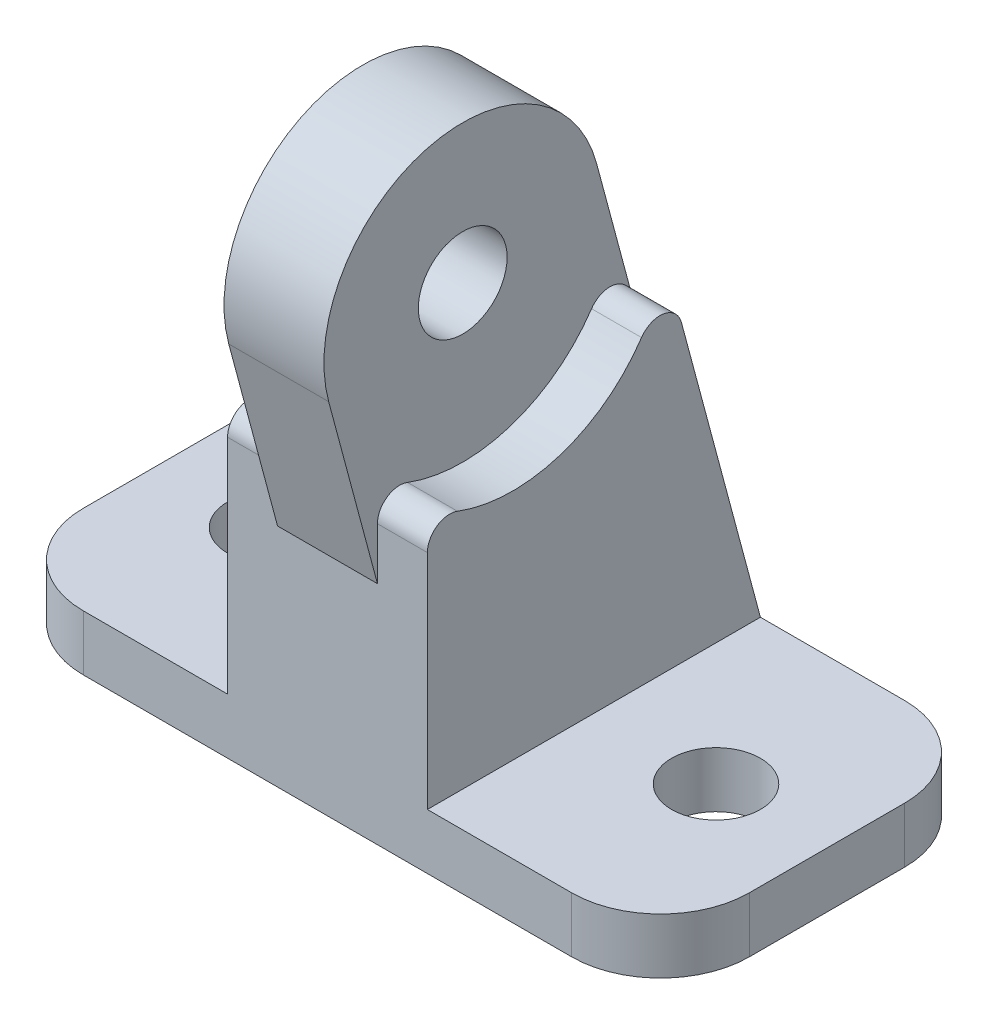
ISO-10303-21;
HEADER;
FILE_DESCRIPTION(('STEP AP214'),'2;1');
FILE_NAME('part.step','',(''),(''),'','','');
FILE_SCHEMA(('AUTOMOTIVE_DESIGN { 1 0 10303 214 1 1 1 1 }'));
ENDSEC;
DATA;
#1=APPLICATION_CONTEXT('core data for automotive mechanical design processes');
#2=APPLICATION_PROTOCOL_DEFINITION('international standard','automotive_design',2000,#1);
#3=PRODUCT_CONTEXT('',#1,'mechanical');
#4=PRODUCT('Part','Part','',(#3));
#5=PRODUCT_RELATED_PRODUCT_CATEGORY('part','',(#4));
#6=PRODUCT_DEFINITION_FORMATION('','',#4);
#7=PRODUCT_DEFINITION_CONTEXT('part definition',#1,'design');
#8=PRODUCT_DEFINITION('design','',#6,#7);
#9=PRODUCT_DEFINITION_SHAPE('','',#8);
#10=(LENGTH_UNIT() NAMED_UNIT(*) SI_UNIT(.MILLI.,.METRE.));
#11=(NAMED_UNIT(*) PLANE_ANGLE_UNIT() SI_UNIT($,.RADIAN.));
#12=(NAMED_UNIT(*) SI_UNIT($,.STERADIAN.) SOLID_ANGLE_UNIT());
#13=UNCERTAINTY_MEASURE_WITH_UNIT(LENGTH_MEASURE(1.E-05),#10,'distance_accuracy_value','');
#14=(GEOMETRIC_REPRESENTATION_CONTEXT(3) GLOBAL_UNCERTAINTY_ASSIGNED_CONTEXT((#13)) GLOBAL_UNIT_ASSIGNED_CONTEXT((#10,
#11,#12)) REPRESENTATION_CONTEXT('',''));
#15=CARTESIAN_POINT('',(0.,0.,0.));
#16=DIRECTION('',(0.,0.,1.));
#17=DIRECTION('',(1.,0.,0.));
#18=AXIS2_PLACEMENT_3D('',#15,#16,#17);
#19=CARTESIAN_POINT('',(-9.,0.,0.));
#20=DIRECTION('',(1.,0.,0.));
#21=DIRECTION('',(0.,0.,-1.));
#22=AXIS2_PLACEMENT_3D('',#19,#20,#21);
#23=PLANE('',#22);
#24=DIRECTION('',(0.,1.,0.));
#25=VECTOR('',#24,1.);
#26=CARTESIAN_POINT('',(-9.,0.,15.));
#27=LINE('',#26,#25);
#28=CARTESIAN_POINT('',(-9.,5.,15.));
#29=VERTEX_POINT('',#28);
#30=CARTESIAN_POINT('',(-9.,25.0424528800157,15.));
#31=VERTEX_POINT('',#30);
#32=EDGE_CURVE('E288',#29,#31,#27,.T.);
#33=ORIENTED_EDGE('',*,*,#32,.T.);
#34=CARTESIAN_POINT('',(-9.,25.0424528800157,13.));
#35=DIRECTION('',(1.,0.,0.));
#36=DIRECTION('',(0.,0.,-1.));
#37=AXIS2_PLACEMENT_3D('',#34,#35,#36);
#38=CIRCLE('',#37,2.);
#39=CARTESIAN_POINT('',(-9.,26.9121462700137,12.2898967487769));
#40=VERTEX_POINT('',#39);
#41=EDGE_CURVE('E277',#40,#31,#38,.T.);
#42=ORIENTED_EDGE('',*,*,#41,.F.);
#43=CARTESIAN_POINT('',(-9.,40.,7.31917399021508));
#44=DIRECTION('',(1.,0.,0.));
#45=DIRECTION('',(0.,0.,-1.));
#46=AXIS2_PLACEMENT_3D('',#43,#44,#45);
#47=CIRCLE('',#46,14.);
#48=CARTESIAN_POINT('',(-9.,32.1742368297092,-4.28933283893913));
#49=VERTEX_POINT('',#48);
#50=EDGE_CURVE('E273',#49,#40,#47,.F.);
#51=ORIENTED_EDGE('',*,*,#50,.F.);
#52=CARTESIAN_POINT('',(-9.,31.0562706625248,-5.94769095738974));
#53=DIRECTION('',(1.,0.,0.));
#54=DIRECTION('',(0.,0.,-1.));
#55=AXIS2_PLACEMENT_3D('',#52,#53,#54);
#56=CIRCLE('',#55,2.);
#57=CARTESIAN_POINT('',(-9.,31.5739087527298,-7.87954260996788));
#58=VERTEX_POINT('',#57);
#59=EDGE_CURVE('E275',#58,#49,#56,.T.);
#60=ORIENTED_EDGE('',*,*,#59,.F.);
#61=DIRECTION('',(0.,0.96592582628907,0.258819045102515));
#62=VECTOR('',#61,1.);
#63=CARTESIAN_POINT('',(-9.,4.0849364905388,-15.2451905283833));
#64=LINE('',#63,#62);
#65=CARTESIAN_POINT('',(-9.,5.,-15.));
#66=VERTEX_POINT('',#65);
#67=EDGE_CURVE('E236',#66,#58,#64,.T.);
#68=ORIENTED_EDGE('',*,*,#67,.F.);
#69=DIRECTION('',(0.,0.,-1.));
#70=VECTOR('',#69,1.);
#71=CARTESIAN_POINT('',(-9.,5.,0.));
#72=LINE('',#71,#70);
#73=EDGE_CURVE('E100',#29,#66,#72,.T.);
#74=ORIENTED_EDGE('',*,*,#73,.F.);
#75=EDGE_LOOP('',(#33,#42,#51,#60,#68,#74));
#76=FACE_BOUND('',#75,.T.);
#77=ADVANCED_FACE('F71',(#76),#23,.F.);
#78=CARTESIAN_POINT('',(9.,0.,0.));
#79=DIRECTION('',(1.,0.,0.));
#80=DIRECTION('',(0.,0.,-1.));
#81=AXIS2_PLACEMENT_3D('',#78,#79,#80);
#82=PLANE('',#81);
#83=CARTESIAN_POINT('',(9.,25.0424528800157,13.));
#84=DIRECTION('',(1.,0.,0.));
#85=DIRECTION('',(0.,0.,-1.));
#86=AXIS2_PLACEMENT_3D('',#83,#84,#85);
#87=CIRCLE('',#86,2.);
#88=CARTESIAN_POINT('',(9.,26.9121462700137,12.2898967487769));
#89=VERTEX_POINT('',#88);
#90=CARTESIAN_POINT('',(9.,25.0424528800157,15.));
#91=VERTEX_POINT('',#90);
#92=EDGE_CURVE('E13',#89,#91,#87,.T.);
#93=ORIENTED_EDGE('',*,*,#92,.T.);
#94=DIRECTION('',(0.,1.,0.));
#95=VECTOR('',#94,1.);
#96=CARTESIAN_POINT('',(9.,0.,15.));
#97=LINE('',#96,#95);
#98=CARTESIAN_POINT('',(9.,5.,15.));
#99=VERTEX_POINT('',#98);
#100=EDGE_CURVE('E285',#99,#91,#97,.T.);
#101=ORIENTED_EDGE('',*,*,#100,.F.);
#102=DIRECTION('',(0.,0.,-1.));
#103=VECTOR('',#102,1.);
#104=CARTESIAN_POINT('',(9.,5.,0.));
#105=LINE('',#104,#103);
#106=CARTESIAN_POINT('',(9.,5.,-15.));
#107=VERTEX_POINT('',#106);
#108=EDGE_CURVE('E282',#99,#107,#105,.T.);
#109=ORIENTED_EDGE('',*,*,#108,.T.);
#110=DIRECTION('',(0.,0.96592582628907,0.258819045102515));
#111=VECTOR('',#110,1.);
#112=CARTESIAN_POINT('',(9.,4.0849364905388,-15.2451905283833));
#113=LINE('',#112,#111);
#114=CARTESIAN_POINT('',(9.,31.5739087527298,-7.87954260996788));
#115=VERTEX_POINT('',#114);
#116=EDGE_CURVE('E276',#107,#115,#113,.T.);
#117=ORIENTED_EDGE('',*,*,#116,.T.);
#118=CARTESIAN_POINT('',(9.,31.0562706625248,-5.94769095738974));
#119=DIRECTION('',(1.,0.,0.));
#120=DIRECTION('',(0.,0.,-1.));
#121=AXIS2_PLACEMENT_3D('',#118,#119,#120);
#122=CIRCLE('',#121,2.);
#123=CARTESIAN_POINT('',(9.,32.1742368297092,-4.28933283893913));
#124=VERTEX_POINT('',#123);
#125=EDGE_CURVE('E373',#115,#124,#122,.T.);
#126=ORIENTED_EDGE('',*,*,#125,.T.);
#127=CARTESIAN_POINT('',(9.,40.,7.31917399021508));
#128=DIRECTION('',(1.,0.,0.));
#129=DIRECTION('',(0.,0.,-1.));
#130=AXIS2_PLACEMENT_3D('',#127,#128,#129);
#131=CIRCLE('',#130,14.);
#132=EDGE_CURVE('E81',#124,#89,#131,.F.);
#133=ORIENTED_EDGE('',*,*,#132,.T.);
#134=EDGE_LOOP('',(#93,#101,#109,#117,#126,#133));
#135=FACE_BOUND('',#134,.T.);
#136=ADVANCED_FACE('F378',(#135),#82,.T.);
#137=CARTESIAN_POINT('',(-22.,5.,7.));
#138=DIRECTION('',(0.,1.,0.));
#139=DIRECTION('',(0.,0.,1.));
#140=AXIS2_PLACEMENT_3D('',#137,#138,#139);
#141=PLANE('',#140);
#142=CARTESIAN_POINT('',(-20.,5.,0.));
#143=DIRECTION('',(0.,1.,0.));
#144=DIRECTION('',(0.,0.,1.));
#145=AXIS2_PLACEMENT_3D('',#142,#143,#144);
#146=CIRCLE('',#145,4.);
#147=CARTESIAN_POINT('',(-20.,5.,4.));
#148=VERTEX_POINT('',#147);
#149=EDGE_CURVE('E306',#148,#148,#146,.T.);
#150=ORIENTED_EDGE('',*,*,#149,.F.);
#151=EDGE_LOOP('',(#150));
#152=FACE_BOUND('',#151,.T.);
#153=DIRECTION('',(1.,0.,0.));
#154=VECTOR('',#153,1.);
#155=CARTESIAN_POINT('',(-22.,5.,15.));
#156=LINE('',#155,#154);
#157=CARTESIAN_POINT('',(-22.,5.,15.));
#158=VERTEX_POINT('',#157);
#159=EDGE_CURVE('E317',#158,#29,#156,.T.);
#160=ORIENTED_EDGE('',*,*,#159,.T.);
#161=ORIENTED_EDGE('',*,*,#73,.T.);
#162=DIRECTION('',(-1.,0.,0.));
#163=VECTOR('',#162,1.);
#164=CARTESIAN_POINT('',(-22.,5.,-15.));
#165=LINE('',#164,#163);
#166=CARTESIAN_POINT('',(-22.,5.,-15.));
#167=VERTEX_POINT('',#166);
#168=EDGE_CURVE('E330',#66,#167,#165,.T.);
#169=ORIENTED_EDGE('',*,*,#168,.T.);
#170=CARTESIAN_POINT('',(-22.,5.,-7.));
#171=DIRECTION('',(0.,1.,0.));
#172=DIRECTION('',(0.,0.,1.));
#173=AXIS2_PLACEMENT_3D('',#170,#171,#172);
#174=CIRCLE('',#173,8.);
#175=CARTESIAN_POINT('',(-30.,5.,-6.99999999999994));
#176=VERTEX_POINT('',#175);
#177=EDGE_CURVE('E329',#167,#176,#174,.T.);
#178=ORIENTED_EDGE('',*,*,#177,.T.);
#179=DIRECTION('',(0.,0.,1.));
#180=VECTOR('',#179,1.);
#181=CARTESIAN_POINT('',(-30.,5.,-6.99999999999994));
#182=LINE('',#181,#180);
#183=CARTESIAN_POINT('',(-30.,5.,6.99999999999995));
#184=VERTEX_POINT('',#183);
#185=EDGE_CURVE('E335',#176,#184,#182,.T.);
#186=ORIENTED_EDGE('',*,*,#185,.T.);
#187=CARTESIAN_POINT('',(-22.,5.,7.));
#188=DIRECTION('',(0.,1.,0.));
#189=DIRECTION('',(0.,0.,1.));
#190=AXIS2_PLACEMENT_3D('',#187,#188,#189);
#191=CIRCLE('',#190,8.);
#192=EDGE_CURVE('E314',#184,#158,#191,.T.);
#193=ORIENTED_EDGE('',*,*,#192,.T.);
#194=EDGE_LOOP('',(#160,#161,#169,#178,#186,#193));
#195=FACE_BOUND('',#194,.T.);
#196=ADVANCED_FACE('F434',(#152,#195),#141,.T.);
#197=ORIENTED_EDGE('',*,*,#108,.F.);
#198=CARTESIAN_POINT('',(21.9999999999999,5.,15.));
#199=VERTEX_POINT('',#198);
#200=EDGE_CURVE('E320',#99,#199,#156,.T.);
#201=ORIENTED_EDGE('',*,*,#200,.T.);
#202=CARTESIAN_POINT('',(22.,5.,7.));
#203=DIRECTION('',(0.,1.,0.));
#204=DIRECTION('',(0.,0.,1.));
#205=AXIS2_PLACEMENT_3D('',#202,#203,#204);
#206=CIRCLE('',#205,8.);
#207=CARTESIAN_POINT('',(30.,5.,6.99999999999995));
#208=VERTEX_POINT('',#207);
#209=EDGE_CURVE('E321',#199,#208,#206,.T.);
#210=ORIENTED_EDGE('',*,*,#209,.T.);
#211=DIRECTION('',(0.,0.,-1.));
#212=VECTOR('',#211,1.);
#213=CARTESIAN_POINT('',(30.,5.,-6.99999999999994));
#214=LINE('',#213,#212);
#215=CARTESIAN_POINT('',(30.,5.,-6.99999999999994));
#216=VERTEX_POINT('',#215);
#217=EDGE_CURVE('E323',#208,#216,#214,.T.);
#218=ORIENTED_EDGE('',*,*,#217,.T.);
#219=CARTESIAN_POINT('',(22.,5.,-7.));
#220=DIRECTION('',(0.,1.,0.));
#221=DIRECTION('',(0.,0.,-1.));
#222=AXIS2_PLACEMENT_3D('',#219,#220,#221);
#223=CIRCLE('',#222,8.);
#224=CARTESIAN_POINT('',(21.9999999999999,5.,-15.));
#225=VERTEX_POINT('',#224);
#226=EDGE_CURVE('E324',#216,#225,#223,.T.);
#227=ORIENTED_EDGE('',*,*,#226,.T.);
#228=EDGE_CURVE('E327',#225,#107,#165,.T.);
#229=ORIENTED_EDGE('',*,*,#228,.T.);
#230=EDGE_LOOP('',(#197,#201,#210,#218,#227,#229));
#231=FACE_BOUND('',#230,.T.);
#232=CARTESIAN_POINT('',(20.,5.,0.));
#233=DIRECTION('',(0.,1.,0.));
#234=DIRECTION('',(0.,0.,1.));
#235=AXIS2_PLACEMENT_3D('',#232,#233,#234);
#236=CIRCLE('',#235,4.);
#237=CARTESIAN_POINT('',(20.,5.,3.99999999999999));
#238=VERTEX_POINT('',#237);
#239=EDGE_CURVE('E301',#238,#238,#236,.T.);
#240=ORIENTED_EDGE('',*,*,#239,.F.);
#241=EDGE_LOOP('',(#240));
#242=FACE_BOUND('',#241,.T.);
#243=ADVANCED_FACE('F451',(#231,#242),#141,.T.);
#244=CARTESIAN_POINT('',(-22.,0.,7.));
#245=DIRECTION('',(0.,1.,0.));
#246=DIRECTION('',(0.,0.,1.));
#247=AXIS2_PLACEMENT_3D('',#244,#245,#246);
#248=PLANE('',#247);
#249=CARTESIAN_POINT('',(-22.,0.,7.));
#250=DIRECTION('',(0.,1.,0.));
#251=DIRECTION('',(0.,0.,1.));
#252=AXIS2_PLACEMENT_3D('',#249,#250,#251);
#253=CIRCLE('',#252,8.);
#254=CARTESIAN_POINT('',(-30.,0.,6.99999999999995));
#255=VERTEX_POINT('',#254);
#256=CARTESIAN_POINT('',(-22.,0.,15.));
#257=VERTEX_POINT('',#256);
#258=EDGE_CURVE('E313',#255,#257,#253,.T.);
#259=ORIENTED_EDGE('',*,*,#258,.F.);
#260=DIRECTION('',(0.,0.,1.));
#261=VECTOR('',#260,1.);
#262=CARTESIAN_POINT('',(-30.,0.,-6.99999999999994));
#263=LINE('',#262,#261);
#264=CARTESIAN_POINT('',(-30.,0.,-6.99999999999994));
#265=VERTEX_POINT('',#264);
#266=EDGE_CURVE('E318',#265,#255,#263,.T.);
#267=ORIENTED_EDGE('',*,*,#266,.F.);
#268=CARTESIAN_POINT('',(-22.,0.,-7.));
#269=DIRECTION('',(0.,1.,0.));
#270=DIRECTION('',(0.,0.,1.));
#271=AXIS2_PLACEMENT_3D('',#268,#269,#270);
#272=CIRCLE('',#271,8.);
#273=CARTESIAN_POINT('',(-22.,0.,-15.));
#274=VERTEX_POINT('',#273);
#275=EDGE_CURVE('E350',#274,#265,#272,.T.);
#276=ORIENTED_EDGE('',*,*,#275,.F.);
#277=DIRECTION('',(-1.,0.,0.));
#278=VECTOR('',#277,1.);
#279=CARTESIAN_POINT('',(-22.,0.,-15.));
#280=LINE('',#279,#278);
#281=CARTESIAN_POINT('',(21.9999999999999,0.,-15.));
#282=VERTEX_POINT('',#281);
#283=EDGE_CURVE('E342',#282,#274,#280,.T.);
#284=ORIENTED_EDGE('',*,*,#283,.F.);
#285=CARTESIAN_POINT('',(22.,0.,-7.));
#286=DIRECTION('',(0.,1.,0.));
#287=DIRECTION('',(0.,0.,-1.));
#288=AXIS2_PLACEMENT_3D('',#285,#286,#287);
#289=CIRCLE('',#288,8.);
#290=CARTESIAN_POINT('',(30.,0.,-6.99999999999994));
#291=VERTEX_POINT('',#290);
#292=EDGE_CURVE('E345',#291,#282,#289,.T.);
#293=ORIENTED_EDGE('',*,*,#292,.F.);
#294=DIRECTION('',(0.,0.,-1.));
#295=VECTOR('',#294,1.);
#296=CARTESIAN_POINT('',(30.,0.,-6.99999999999994));
#297=LINE('',#296,#295);
#298=CARTESIAN_POINT('',(30.,0.,6.99999999999995));
#299=VERTEX_POINT('',#298);
#300=EDGE_CURVE('E344',#299,#291,#297,.T.);
#301=ORIENTED_EDGE('',*,*,#300,.F.);
#302=CARTESIAN_POINT('',(22.,0.,7.));
#303=DIRECTION('',(0.,1.,0.));
#304=DIRECTION('',(0.,0.,1.));
#305=AXIS2_PLACEMENT_3D('',#302,#303,#304);
#306=CIRCLE('',#305,8.);
#307=CARTESIAN_POINT('',(21.9999999999999,0.,15.));
#308=VERTEX_POINT('',#307);
#309=EDGE_CURVE('E337',#308,#299,#306,.T.);
#310=ORIENTED_EDGE('',*,*,#309,.F.);
#311=DIRECTION('',(1.,0.,0.));
#312=VECTOR('',#311,1.);
#313=CARTESIAN_POINT('',(-22.,0.,15.));
#314=LINE('',#313,#312);
#315=EDGE_CURVE('E340',#257,#308,#314,.T.);
#316=ORIENTED_EDGE('',*,*,#315,.F.);
#317=EDGE_LOOP('',(#259,#267,#276,#284,#293,#301,#310,#316));
#318=FACE_BOUND('',#317,.T.);
#319=CARTESIAN_POINT('',(-20.,0.,0.));
#320=DIRECTION('',(0.,1.,0.));
#321=DIRECTION('',(0.,0.,1.));
#322=AXIS2_PLACEMENT_3D('',#319,#320,#321);
#323=CIRCLE('',#322,4.);
#324=CARTESIAN_POINT('',(-20.,0.,4.));
#325=VERTEX_POINT('',#324);
#326=EDGE_CURVE('E302',#325,#325,#323,.T.);
#327=ORIENTED_EDGE('',*,*,#326,.T.);
#328=EDGE_LOOP('',(#327));
#329=FACE_BOUND('',#328,.T.);
#330=CARTESIAN_POINT('',(20.,0.,0.));
#331=DIRECTION('',(0.,1.,0.));
#332=DIRECTION('',(0.,0.,1.));
#333=AXIS2_PLACEMENT_3D('',#330,#331,#332);
#334=CIRCLE('',#333,4.);
#335=CARTESIAN_POINT('',(20.,0.,3.99999999999999));
#336=VERTEX_POINT('',#335);
#337=EDGE_CURVE('E304',#336,#336,#334,.T.);
#338=ORIENTED_EDGE('',*,*,#337,.T.);
#339=EDGE_LOOP('',(#338));
#340=FACE_BOUND('',#339,.T.);
#341=ADVANCED_FACE('F445',(#318,#329,#340),#248,.F.);
#342=CARTESIAN_POINT('',(-22.,5.,7.));
#343=DIRECTION('',(0.,-1.,0.));
#344=DIRECTION('',(0.,0.,-1.));
#345=AXIS2_PLACEMENT_3D('',#342,#343,#344);
#346=CYLINDRICAL_SURFACE('',#345,8.);
#347=ORIENTED_EDGE('',*,*,#258,.T.);
#348=DIRECTION('',(0.,-1.,0.));
#349=VECTOR('',#348,1.);
#350=CARTESIAN_POINT('',(-22.,5.,15.));
#351=LINE('',#350,#349);
#352=EDGE_CURVE('E367',#158,#257,#351,.T.);
#353=ORIENTED_EDGE('',*,*,#352,.F.);
#354=ORIENTED_EDGE('',*,*,#192,.F.);
#355=DIRECTION('',(0.,-1.,0.));
#356=VECTOR('',#355,1.);
#357=CARTESIAN_POINT('',(-30.,5.,6.99999999999995));
#358=LINE('',#357,#356);
#359=EDGE_CURVE('E331',#184,#255,#358,.T.);
#360=ORIENTED_EDGE('',*,*,#359,.T.);
#361=EDGE_LOOP('',(#347,#353,#354,#360));
#362=FACE_BOUND('',#361,.T.);
#363=ADVANCED_FACE('F73',(#362),#346,.T.);
#364=CARTESIAN_POINT('',(-22.,5.,15.));
#365=DIRECTION('',(0.,0.,-1.));
#366=DIRECTION('',(-1.,0.,0.));
#367=AXIS2_PLACEMENT_3D('',#364,#365,#366);
#368=PLANE('',#367);
#369=ORIENTED_EDGE('',*,*,#315,.T.);
#370=DIRECTION('',(0.,-1.,0.));
#371=VECTOR('',#370,1.);
#372=CARTESIAN_POINT('',(21.9999999999999,5.,15.));
#373=LINE('',#372,#371);
#374=EDGE_CURVE('E370',#199,#308,#373,.T.);
#375=ORIENTED_EDGE('',*,*,#374,.F.);
#376=ORIENTED_EDGE('',*,*,#200,.F.);
#377=ORIENTED_EDGE('',*,*,#100,.T.);
#378=DIRECTION('',(1.,0.,0.));
#379=VECTOR('',#378,1.);
#380=CARTESIAN_POINT('',(-42.4219732605604,25.0424528800157,15.));
#381=LINE('',#380,#379);
#382=CARTESIAN_POINT('',(4.5,25.0424528800157,15.));
#383=VERTEX_POINT('',#382);
#384=EDGE_CURVE('E234',#383,#91,#381,.T.);
#385=ORIENTED_EDGE('',*,*,#384,.F.);
#386=DIRECTION('',(0.,-1.,0.));
#387=VECTOR('',#386,1.);
#388=CARTESIAN_POINT('',(4.5,20.36894159816,15.));
#389=LINE('',#388,#387);
#390=CARTESIAN_POINT('',(4.5,20.36894159816,15.));
#391=VERTEX_POINT('',#390);
#392=EDGE_CURVE('E242',#383,#391,#389,.T.);
#393=ORIENTED_EDGE('',*,*,#392,.T.);
#394=DIRECTION('',(-1.,0.,0.));
#395=VECTOR('',#394,1.);
#396=CARTESIAN_POINT('',(9.,20.36894159816,15.));
#397=LINE('',#396,#395);
#398=CARTESIAN_POINT('',(-4.5,20.36894159816,15.));
#399=VERTEX_POINT('',#398);
#400=EDGE_CURVE('E291',#391,#399,#397,.T.);
#401=ORIENTED_EDGE('',*,*,#400,.T.);
#402=DIRECTION('',(0.,1.,0.));
#403=VECTOR('',#402,1.);
#404=CARTESIAN_POINT('',(-4.5,20.36894159816,15.));
#405=LINE('',#404,#403);
#406=CARTESIAN_POINT('',(-4.5,25.0424528800157,15.));
#407=VERTEX_POINT('',#406);
#408=EDGE_CURVE('E415',#399,#407,#405,.T.);
#409=ORIENTED_EDGE('',*,*,#408,.T.);
#410=DIRECTION('',(-1.,0.,0.));
#411=VECTOR('',#410,1.);
#412=CARTESIAN_POINT('',(42.4219732605604,25.0424528800157,15.));
#413=LINE('',#412,#411);
#414=EDGE_CURVE('E418',#407,#31,#413,.T.);
#415=ORIENTED_EDGE('',*,*,#414,.T.);
#416=ORIENTED_EDGE('',*,*,#32,.F.);
#417=ORIENTED_EDGE('',*,*,#159,.F.);
#418=ORIENTED_EDGE('',*,*,#352,.T.);
#419=EDGE_LOOP('',(#369,#375,#376,#377,#385,#393,#401,#409,#415,#416,#417,#418));
#420=FACE_BOUND('',#419,.T.);
#421=ADVANCED_FACE('F396',(#420),#368,.F.);
#422=CARTESIAN_POINT('',(22.,5.,7.));
#423=DIRECTION('',(0.,-1.,0.));
#424=DIRECTION('',(0.,0.,-1.));
#425=AXIS2_PLACEMENT_3D('',#422,#423,#424);
#426=CYLINDRICAL_SURFACE('',#425,8.);
#427=ORIENTED_EDGE('',*,*,#309,.T.);
#428=DIRECTION('',(0.,-1.,0.));
#429=VECTOR('',#428,1.);
#430=CARTESIAN_POINT('',(30.,5.,6.99999999999995));
#431=LINE('',#430,#429);
#432=EDGE_CURVE('E365',#208,#299,#431,.T.);
#433=ORIENTED_EDGE('',*,*,#432,.F.);
#434=ORIENTED_EDGE('',*,*,#209,.F.);
#435=ORIENTED_EDGE('',*,*,#374,.T.);
#436=EDGE_LOOP('',(#427,#433,#434,#435));
#437=FACE_BOUND('',#436,.T.);
#438=ADVANCED_FACE('F447',(#437),#426,.T.);
#439=CARTESIAN_POINT('',(30.,5.,-6.99999999999994));
#440=DIRECTION('',(-1.,0.,0.));
#441=DIRECTION('',(0.,0.,1.));
#442=AXIS2_PLACEMENT_3D('',#439,#440,#441);
#443=PLANE('',#442);
#444=ORIENTED_EDGE('',*,*,#300,.T.);
#445=DIRECTION('',(0.,-1.,0.));
#446=VECTOR('',#445,1.);
#447=CARTESIAN_POINT('',(30.,5.,-6.99999999999994));
#448=LINE('',#447,#446);
#449=EDGE_CURVE('E363',#216,#291,#448,.T.);
#450=ORIENTED_EDGE('',*,*,#449,.F.);
#451=ORIENTED_EDGE('',*,*,#217,.F.);
#452=ORIENTED_EDGE('',*,*,#432,.T.);
#453=EDGE_LOOP('',(#444,#450,#451,#452));
#454=FACE_BOUND('',#453,.T.);
#455=ADVANCED_FACE('F456',(#454),#443,.F.);
#456=CARTESIAN_POINT('',(22.,5.,-7.));
#457=DIRECTION('',(0.,-1.,0.));
#458=DIRECTION('',(0.,0.,-1.));
#459=AXIS2_PLACEMENT_3D('',#456,#457,#458);
#460=CYLINDRICAL_SURFACE('',#459,8.);
#461=ORIENTED_EDGE('',*,*,#292,.T.);
#462=DIRECTION('',(0.,-1.,0.));
#463=VECTOR('',#462,1.);
#464=CARTESIAN_POINT('',(21.9999999999999,5.,-15.));
#465=LINE('',#464,#463);
#466=EDGE_CURVE('E360',#225,#282,#465,.T.);
#467=ORIENTED_EDGE('',*,*,#466,.F.);
#468=ORIENTED_EDGE('',*,*,#226,.F.);
#469=ORIENTED_EDGE('',*,*,#449,.T.);
#470=EDGE_LOOP('',(#461,#467,#468,#469));
#471=FACE_BOUND('',#470,.T.);
#472=ADVANCED_FACE('F463',(#471),#460,.T.);
#473=CARTESIAN_POINT('',(-22.,5.,-15.));
#474=DIRECTION('',(0.,0.,1.));
#475=DIRECTION('',(1.,0.,0.));
#476=AXIS2_PLACEMENT_3D('',#473,#474,#475);
#477=PLANE('',#476);
#478=ORIENTED_EDGE('',*,*,#283,.T.);
#479=DIRECTION('',(0.,-1.,0.));
#480=VECTOR('',#479,1.);
#481=CARTESIAN_POINT('',(-22.,5.,-15.));
#482=LINE('',#481,#480);
#483=EDGE_CURVE('E354',#167,#274,#482,.T.);
#484=ORIENTED_EDGE('',*,*,#483,.F.);
#485=ORIENTED_EDGE('',*,*,#168,.F.);
#486=DIRECTION('',(-1.,0.,0.));
#487=VECTOR('',#486,1.);
#488=CARTESIAN_POINT('',(9.,5.,-15.));
#489=LINE('',#488,#487);
#490=EDGE_CURVE('E286',#107,#66,#489,.T.);
#491=ORIENTED_EDGE('',*,*,#490,.F.);
#492=ORIENTED_EDGE('',*,*,#228,.F.);
#493=ORIENTED_EDGE('',*,*,#466,.T.);
#494=EDGE_LOOP('',(#478,#484,#485,#491,#492,#493));
#495=FACE_BOUND('',#494,.T.);
#496=ADVANCED_FACE('F464',(#495),#477,.F.);
#497=CARTESIAN_POINT('',(-22.,5.,-7.));
#498=DIRECTION('',(0.,-1.,0.));
#499=DIRECTION('',(0.,0.,-1.));
#500=AXIS2_PLACEMENT_3D('',#497,#498,#499);
#501=CYLINDRICAL_SURFACE('',#500,8.);
#502=ORIENTED_EDGE('',*,*,#275,.T.);
#503=DIRECTION('',(0.,-1.,0.));
#504=VECTOR('',#503,1.);
#505=CARTESIAN_POINT('',(-30.,5.,-6.99999999999994));
#506=LINE('',#505,#504);
#507=EDGE_CURVE('E355',#176,#265,#506,.T.);
#508=ORIENTED_EDGE('',*,*,#507,.F.);
#509=ORIENTED_EDGE('',*,*,#177,.F.);
#510=ORIENTED_EDGE('',*,*,#483,.T.);
#511=EDGE_LOOP('',(#502,#508,#509,#510));
#512=FACE_BOUND('',#511,.T.);
#513=ADVANCED_FACE('F467',(#512),#501,.T.);
#514=CARTESIAN_POINT('',(-30.,5.,-6.99999999999994));
#515=DIRECTION('',(1.,0.,0.));
#516=DIRECTION('',(0.,0.,-1.));
#517=AXIS2_PLACEMENT_3D('',#514,#515,#516);
#518=PLANE('',#517);
#519=ORIENTED_EDGE('',*,*,#266,.T.);
#520=ORIENTED_EDGE('',*,*,#359,.F.);
#521=ORIENTED_EDGE('',*,*,#185,.F.);
#522=ORIENTED_EDGE('',*,*,#507,.T.);
#523=EDGE_LOOP('',(#519,#520,#521,#522));
#524=FACE_BOUND('',#523,.T.);
#525=ADVANCED_FACE('F472',(#524),#518,.F.);
#526=CARTESIAN_POINT('',(-20.,5.,0.));
#527=DIRECTION('',(0.,-1.,0.));
#528=DIRECTION('',(0.,0.,-1.));
#529=AXIS2_PLACEMENT_3D('',#526,#527,#528);
#530=CYLINDRICAL_SURFACE('',#529,4.);
#531=ORIENTED_EDGE('',*,*,#149,.T.);
#532=EDGE_LOOP('',(#531));
#533=FACE_BOUND('',#532,.T.);
#534=ORIENTED_EDGE('',*,*,#326,.F.);
#535=EDGE_LOOP('',(#534));
#536=FACE_BOUND('',#535,.T.);
#537=ADVANCED_FACE('F475',(#533,#536),#530,.F.);
#538=CARTESIAN_POINT('',(20.,5.,0.));
#539=DIRECTION('',(0.,-1.,0.));
#540=DIRECTION('',(0.,0.,-1.));
#541=AXIS2_PLACEMENT_3D('',#538,#539,#540);
#542=CYLINDRICAL_SURFACE('',#541,4.);
#543=ORIENTED_EDGE('',*,*,#239,.T.);
#544=EDGE_LOOP('',(#543));
#545=FACE_BOUND('',#544,.T.);
#546=ORIENTED_EDGE('',*,*,#337,.F.);
#547=EDGE_LOOP('',(#546));
#548=FACE_BOUND('',#547,.T.);
#549=ADVANCED_FACE('F477',(#545,#548),#542,.F.);
#550=CARTESIAN_POINT('',(9.,-2.38553963702406,8.90295512884346));
#551=DIRECTION('',(0.,0.258819045102514,-0.96592582628907));
#552=DIRECTION('',(0.,0.96592582628907,0.258819045102514));
#553=AXIS2_PLACEMENT_3D('',#550,#551,#552);
#554=PLANE('',#553);
#555=DIRECTION('',(-1.,0.,0.));
#556=VECTOR('',#555,1.);
#557=CARTESIAN_POINT('',(9.,36.7647619362186,19.3932468188284));
#558=LINE('',#557,#556);
#559=CARTESIAN_POINT('',(4.5,36.7647619362186,19.3932468188285));
#560=VERTEX_POINT('',#559);
#561=CARTESIAN_POINT('',(-4.5,36.7647619362186,19.3932468188285));
#562=VERTEX_POINT('',#561);
#563=EDGE_CURVE('E298',#560,#562,#558,.T.);
#564=ORIENTED_EDGE('',*,*,#563,.T.);
#565=DIRECTION('',(0.,-0.96592582628907,-0.258819045102515));
#566=VECTOR('',#565,1.);
#567=CARTESIAN_POINT('',(-4.5,36.7647619362186,19.3932468188285));
#568=LINE('',#567,#566);
#569=EDGE_CURVE('E409',#562,#399,#568,.T.);
#570=ORIENTED_EDGE('',*,*,#569,.T.);
#571=ORIENTED_EDGE('',*,*,#400,.F.);
#572=DIRECTION('',(0.,0.96592582628907,0.258819045102515));
#573=VECTOR('',#572,1.);
#574=CARTESIAN_POINT('',(4.5,36.7647619362186,19.3932468188285));
#575=LINE('',#574,#573);
#576=EDGE_CURVE('E259',#391,#560,#575,.T.);
#577=ORIENTED_EDGE('',*,*,#576,.T.);
#578=EDGE_LOOP('',(#564,#570,#571,#577));
#579=FACE_BOUND('',#578,.T.);
#580=ADVANCED_FACE('F406',(#579),#554,.F.);
#581=CARTESIAN_POINT('',(9.,40.,7.31917399021508));
#582=DIRECTION('',(-1.,0.,0.));
#583=DIRECTION('',(0.,0.,1.));
#584=AXIS2_PLACEMENT_3D('',#581,#582,#583);
#585=CYLINDRICAL_SURFACE('',#584,12.5);
#586=DIRECTION('',(-1.,0.,0.));
#587=VECTOR('',#586,1.);
#588=CARTESIAN_POINT('',(9.,43.2352380637814,-4.7548988383983));
#589=LINE('',#588,#587);
#590=CARTESIAN_POINT('',(4.5,43.2352380637814,-4.7548988383983));
#591=VERTEX_POINT('',#590);
#592=CARTESIAN_POINT('',(-4.5,43.2352380637814,-4.7548988383983));
#593=VERTEX_POINT('',#592);
#594=EDGE_CURVE('E297',#591,#593,#589,.T.);
#595=ORIENTED_EDGE('',*,*,#594,.T.);
#596=CARTESIAN_POINT('',(-4.5,40.,7.31917399021508));
#597=DIRECTION('',(1.,0.,0.));
#598=DIRECTION('',(0.,0.,-1.));
#599=AXIS2_PLACEMENT_3D('',#596,#597,#598);
#600=CIRCLE('',#599,12.5);
#601=EDGE_CURVE('E225',#593,#562,#600,.T.);
#602=ORIENTED_EDGE('',*,*,#601,.T.);
#603=ORIENTED_EDGE('',*,*,#563,.F.);
#604=CARTESIAN_POINT('',(4.5,40.,7.31917399021508));
#605=DIRECTION('',(1.,0.,0.));
#606=DIRECTION('',(0.,0.,-1.));
#607=AXIS2_PLACEMENT_3D('',#604,#605,#606);
#608=CIRCLE('',#607,12.5);
#609=EDGE_CURVE('E258',#560,#591,#608,.F.);
#610=ORIENTED_EDGE('',*,*,#609,.T.);
#611=EDGE_LOOP('',(#595,#602,#603,#610));
#612=FACE_BOUND('',#611,.T.);
#613=ADVANCED_FACE('F403',(#612),#585,.T.);
#614=CARTESIAN_POINT('',(9.,4.0849364905388,-15.2451905283833));
#615=DIRECTION('',(0.,-0.258819045102514,0.96592582628907));
#616=DIRECTION('',(0.,-0.96592582628907,-0.258819045102514));
#617=AXIS2_PLACEMENT_3D('',#614,#615,#616);
#618=PLANE('',#617);
#619=DIRECTION('',(-1.,0.,0.));
#620=VECTOR('',#619,1.);
#621=CARTESIAN_POINT('',(42.4219732605604,31.5739087527298,-7.87954260996788));
#622=LINE('',#621,#620);
#623=CARTESIAN_POINT('',(-4.5,31.5739087527298,-7.87954260996788));
#624=VERTEX_POINT('',#623);
#625=EDGE_CURVE('E90',#624,#58,#622,.T.);
#626=ORIENTED_EDGE('',*,*,#625,.F.);
#627=DIRECTION('',(0.,0.96592582628907,0.258819045102514));
#628=VECTOR('',#627,1.);
#629=CARTESIAN_POINT('',(-4.5,31.5739087527298,-7.87954260996788));
#630=LINE('',#629,#628);
#631=EDGE_CURVE('E220',#624,#593,#630,.T.);
#632=ORIENTED_EDGE('',*,*,#631,.T.);
#633=ORIENTED_EDGE('',*,*,#594,.F.);
#634=DIRECTION('',(0.,-0.96592582628907,-0.258819045102514));
#635=VECTOR('',#634,1.);
#636=CARTESIAN_POINT('',(4.5,31.5739087527298,-7.87954260996788));
#637=LINE('',#636,#635);
#638=CARTESIAN_POINT('',(4.5,31.5739087527298,-7.87954260996788));
#639=VERTEX_POINT('',#638);
#640=EDGE_CURVE('E251',#591,#639,#637,.T.);
#641=ORIENTED_EDGE('',*,*,#640,.T.);
#642=DIRECTION('',(1.,0.,0.));
#643=VECTOR('',#642,1.);
#644=CARTESIAN_POINT('',(-42.4219732605604,31.5739087527298,-7.87954260996788));
#645=LINE('',#644,#643);
#646=EDGE_CURVE('E246',#639,#115,#645,.T.);
#647=ORIENTED_EDGE('',*,*,#646,.T.);
#648=ORIENTED_EDGE('',*,*,#116,.F.);
#649=ORIENTED_EDGE('',*,*,#490,.T.);
#650=ORIENTED_EDGE('',*,*,#67,.T.);
#651=EDGE_LOOP('',(#626,#632,#633,#641,#647,#648,#649,#650));
#652=FACE_BOUND('',#651,.T.);
#653=ADVANCED_FACE('F232',(#652),#618,.F.);
#654=CARTESIAN_POINT('',(-42.4219732605604,40.,7.31917399021508));
#655=DIRECTION('',(1.,0.,0.));
#656=DIRECTION('',(0.,0.,-1.));
#657=AXIS2_PLACEMENT_3D('',#654,#655,#656);
#658=CYLINDRICAL_SURFACE('',#657,14.);
#659=DIRECTION('',(1.,0.,0.));
#660=VECTOR('',#659,1.);
#661=CARTESIAN_POINT('',(-42.4219732605604,32.1742368297092,-4.28933283893913));
#662=LINE('',#661,#660);
#663=CARTESIAN_POINT('',(4.5,32.1742368297092,-4.28933283893913));
#664=VERTEX_POINT('',#663);
#665=EDGE_CURVE('E265',#664,#124,#662,.T.);
#666=ORIENTED_EDGE('',*,*,#665,.F.);
#667=CARTESIAN_POINT('',(4.5,40.,7.31917399021508));
#668=DIRECTION('',(1.,0.,0.));
#669=DIRECTION('',(0.,0.,-1.));
#670=AXIS2_PLACEMENT_3D('',#667,#668,#669);
#671=CIRCLE('',#670,14.);
#672=CARTESIAN_POINT('',(4.5,26.9121462700137,12.2898967487769));
#673=VERTEX_POINT('',#672);
#674=EDGE_CURVE('E248',#664,#673,#671,.F.);
#675=ORIENTED_EDGE('',*,*,#674,.T.);
#676=DIRECTION('',(1.,0.,0.));
#677=VECTOR('',#676,1.);
#678=CARTESIAN_POINT('',(-42.4219732605604,26.9121462700137,12.2898967487769));
#679=LINE('',#678,#677);
#680=EDGE_CURVE('E264',#673,#89,#679,.T.);
#681=ORIENTED_EDGE('',*,*,#680,.T.);
#682=ORIENTED_EDGE('',*,*,#132,.F.);
#683=EDGE_LOOP('',(#666,#675,#681,#682));
#684=FACE_BOUND('',#683,.T.);
#685=ADVANCED_FACE('F385',(#684),#658,.F.);
#686=CARTESIAN_POINT('',(-42.4219732605604,25.0424528800157,13.));
#687=DIRECTION('',(1.,0.,0.));
#688=DIRECTION('',(0.,0.,-1.));
#689=AXIS2_PLACEMENT_3D('',#686,#687,#688);
#690=CYLINDRICAL_SURFACE('',#689,2.);
#691=ORIENTED_EDGE('',*,*,#680,.F.);
#692=CARTESIAN_POINT('',(4.5,25.0424528800157,13.));
#693=DIRECTION('',(1.,0.,0.));
#694=DIRECTION('',(0.,0.,-1.));
#695=AXIS2_PLACEMENT_3D('',#692,#693,#694);
#696=CIRCLE('',#695,2.);
#697=EDGE_CURVE('E249',#673,#383,#696,.T.);
#698=ORIENTED_EDGE('',*,*,#697,.T.);
#699=ORIENTED_EDGE('',*,*,#384,.T.);
#700=ORIENTED_EDGE('',*,*,#92,.F.);
#701=EDGE_LOOP('',(#691,#698,#699,#700));
#702=FACE_BOUND('',#701,.T.);
#703=ADVANCED_FACE('F394',(#702),#690,.T.);
#704=CARTESIAN_POINT('',(-42.4219732605604,31.0562706625248,-5.94769095738974));
#705=DIRECTION('',(1.,0.,0.));
#706=DIRECTION('',(0.,0.,-1.));
#707=AXIS2_PLACEMENT_3D('',#704,#705,#706);
#708=CYLINDRICAL_SURFACE('',#707,2.);
#709=ORIENTED_EDGE('',*,*,#646,.F.);
#710=CARTESIAN_POINT('',(4.5,31.0562706625248,-5.94769095738974));
#711=DIRECTION('',(1.,0.,0.));
#712=DIRECTION('',(0.,0.,-1.));
#713=AXIS2_PLACEMENT_3D('',#710,#711,#712);
#714=CIRCLE('',#713,2.);
#715=EDGE_CURVE('E253',#639,#664,#714,.T.);
#716=ORIENTED_EDGE('',*,*,#715,.T.);
#717=ORIENTED_EDGE('',*,*,#665,.T.);
#718=ORIENTED_EDGE('',*,*,#125,.F.);
#719=EDGE_LOOP('',(#709,#716,#717,#718));
#720=FACE_BOUND('',#719,.T.);
#721=ADVANCED_FACE('F387',(#720),#708,.T.);
#722=CARTESIAN_POINT('',(4.5,0.,0.));
#723=DIRECTION('',(1.,0.,0.));
#724=DIRECTION('',(0.,0.,-1.));
#725=AXIS2_PLACEMENT_3D('',#722,#723,#724);
#726=PLANE('',#725);
#727=CARTESIAN_POINT('',(4.5,40.,7.31917399021508));
#728=DIRECTION('',(1.,0.,0.));
#729=DIRECTION('',(0.,0.,-1.));
#730=AXIS2_PLACEMENT_3D('',#727,#728,#729);
#731=CIRCLE('',#730,4.);
#732=CARTESIAN_POINT('',(4.5,40.,3.31917399021508));
#733=VERTEX_POINT('',#732);
#734=EDGE_CURVE('E618',#733,#733,#731,.T.);
#735=ORIENTED_EDGE('',*,*,#734,.F.);
#736=EDGE_LOOP('',(#735));
#737=FACE_BOUND('',#736,.T.);
#738=ORIENTED_EDGE('',*,*,#609,.F.);
#739=ORIENTED_EDGE('',*,*,#576,.F.);
#740=ORIENTED_EDGE('',*,*,#392,.F.);
#741=ORIENTED_EDGE('',*,*,#697,.F.);
#742=ORIENTED_EDGE('',*,*,#674,.F.);
#743=ORIENTED_EDGE('',*,*,#715,.F.);
#744=ORIENTED_EDGE('',*,*,#640,.F.);
#745=EDGE_LOOP('',(#738,#739,#740,#741,#742,#743,#744));
#746=FACE_BOUND('',#745,.T.);
#747=ADVANCED_FACE('F388',(#737,#746),#726,.T.);
#748=CARTESIAN_POINT('',(42.4219732605604,25.0424528800157,13.));
#749=DIRECTION('',(-1.,0.,0.));
#750=DIRECTION('',(0.,0.,1.));
#751=AXIS2_PLACEMENT_3D('',#748,#749,#750);
#752=CYLINDRICAL_SURFACE('',#751,2.);
#753=ORIENTED_EDGE('',*,*,#41,.T.);
#754=ORIENTED_EDGE('',*,*,#414,.F.);
#755=CARTESIAN_POINT('',(-4.5,25.0424528800157,13.));
#756=DIRECTION('',(1.,0.,0.));
#757=DIRECTION('',(0.,0.,-1.));
#758=AXIS2_PLACEMENT_3D('',#755,#756,#757);
#759=CIRCLE('',#758,2.);
#760=CARTESIAN_POINT('',(-4.5,26.9121462700137,12.2898967487769));
#761=VERTEX_POINT('',#760);
#762=EDGE_CURVE('E417',#407,#761,#759,.F.);
#763=ORIENTED_EDGE('',*,*,#762,.T.);
#764=DIRECTION('',(-1.,0.,0.));
#765=VECTOR('',#764,1.);
#766=CARTESIAN_POINT('',(42.4219732605604,26.9121462700137,12.2898967487769));
#767=LINE('',#766,#765);
#768=EDGE_CURVE('E238',#761,#40,#767,.T.);
#769=ORIENTED_EDGE('',*,*,#768,.T.);
#770=EDGE_LOOP('',(#753,#754,#763,#769));
#771=FACE_BOUND('',#770,.T.);
#772=ADVANCED_FACE('F427',(#771),#752,.T.);
#773=CARTESIAN_POINT('',(42.4219732605604,40.,7.31917399021508));
#774=DIRECTION('',(-1.,0.,0.));
#775=DIRECTION('',(0.,0.,1.));
#776=AXIS2_PLACEMENT_3D('',#773,#774,#775);
#777=CYLINDRICAL_SURFACE('',#776,14.);
#778=ORIENTED_EDGE('',*,*,#50,.T.);
#779=ORIENTED_EDGE('',*,*,#768,.F.);
#780=CARTESIAN_POINT('',(-4.5,40.,7.31917399021508));
#781=DIRECTION('',(1.,0.,0.));
#782=DIRECTION('',(0.,0.,-1.));
#783=AXIS2_PLACEMENT_3D('',#780,#781,#782);
#784=CIRCLE('',#783,14.);
#785=CARTESIAN_POINT('',(-4.5,32.1742368297092,-4.28933283893913));
#786=VERTEX_POINT('',#785);
#787=EDGE_CURVE('E231',#761,#786,#784,.T.);
#788=ORIENTED_EDGE('',*,*,#787,.T.);
#789=DIRECTION('',(-1.,0.,0.));
#790=VECTOR('',#789,1.);
#791=CARTESIAN_POINT('',(42.4219732605604,32.1742368297092,-4.28933283893913));
#792=LINE('',#791,#790);
#793=EDGE_CURVE('E227',#786,#49,#792,.T.);
#794=ORIENTED_EDGE('',*,*,#793,.T.);
#795=EDGE_LOOP('',(#778,#779,#788,#794));
#796=FACE_BOUND('',#795,.T.);
#797=ADVANCED_FACE('F577',(#796),#777,.F.);
#798=CARTESIAN_POINT('',(42.4219732605604,31.0562706625248,-5.94769095738974));
#799=DIRECTION('',(-1.,0.,0.));
#800=DIRECTION('',(0.,0.,1.));
#801=AXIS2_PLACEMENT_3D('',#798,#799,#800);
#802=CYLINDRICAL_SURFACE('',#801,2.);
#803=ORIENTED_EDGE('',*,*,#59,.T.);
#804=ORIENTED_EDGE('',*,*,#793,.F.);
#805=CARTESIAN_POINT('',(-4.5,31.0562706625248,-5.94769095738974));
#806=DIRECTION('',(1.,0.,0.));
#807=DIRECTION('',(0.,0.,-1.));
#808=AXIS2_PLACEMENT_3D('',#805,#806,#807);
#809=CIRCLE('',#808,2.);
#810=EDGE_CURVE('E218',#786,#624,#809,.F.);
#811=ORIENTED_EDGE('',*,*,#810,.T.);
#812=ORIENTED_EDGE('',*,*,#625,.T.);
#813=EDGE_LOOP('',(#803,#804,#811,#812));
#814=FACE_BOUND('',#813,.T.);
#815=ADVANCED_FACE('F230',(#814),#802,.T.);
#816=CARTESIAN_POINT('',(-4.5,0.,0.));
#817=DIRECTION('',(1.,0.,0.));
#818=DIRECTION('',(0.,0.,-1.));
#819=AXIS2_PLACEMENT_3D('',#816,#817,#818);
#820=PLANE('',#819);
#821=CARTESIAN_POINT('',(-4.5,40.,7.31917399021508));
#822=DIRECTION('',(1.,0.,0.));
#823=DIRECTION('',(0.,0.,-1.));
#824=AXIS2_PLACEMENT_3D('',#821,#822,#823);
#825=CIRCLE('',#824,4.);
#826=CARTESIAN_POINT('',(-4.5,40.,3.31917399021508));
#827=VERTEX_POINT('',#826);
#828=EDGE_CURVE('E80',#827,#827,#825,.T.);
#829=ORIENTED_EDGE('',*,*,#828,.T.);
#830=EDGE_LOOP('',(#829));
#831=FACE_BOUND('',#830,.T.);
#832=ORIENTED_EDGE('',*,*,#631,.F.);
#833=ORIENTED_EDGE('',*,*,#810,.F.);
#834=ORIENTED_EDGE('',*,*,#787,.F.);
#835=ORIENTED_EDGE('',*,*,#762,.F.);
#836=ORIENTED_EDGE('',*,*,#408,.F.);
#837=ORIENTED_EDGE('',*,*,#569,.F.);
#838=ORIENTED_EDGE('',*,*,#601,.F.);
#839=EDGE_LOOP('',(#832,#833,#834,#835,#836,#837,#838));
#840=FACE_BOUND('',#839,.T.);
#841=ADVANCED_FACE('F217',(#831,#840),#820,.F.);
#842=CARTESIAN_POINT('',(-30.,40.,7.31917399021508));
#843=DIRECTION('',(1.,0.,0.));
#844=DIRECTION('',(0.,0.,-1.));
#845=AXIS2_PLACEMENT_3D('',#842,#843,#844);
#846=CYLINDRICAL_SURFACE('',#845,4.);
#847=ORIENTED_EDGE('',*,*,#734,.T.);
#848=EDGE_LOOP('',(#847));
#849=FACE_BOUND('',#848,.T.);
#850=ORIENTED_EDGE('',*,*,#828,.F.);
#851=EDGE_LOOP('',(#850));
#852=FACE_BOUND('',#851,.T.);
#853=ADVANCED_FACE('F602',(#849,#852),#846,.F.);
#854=CLOSED_SHELL('',(#77,#136,#196,#243,#341,#363,#421,#438,#455,#472,#496,#513,#525,#537,#549,
#580,#613,#653,#685,#703,#721,#747,#772,#797,#815,#841,#853));
#855=MANIFOLD_SOLID_BREP('B2',#854);
#856=ADVANCED_BREP_SHAPE_REPRESENTATION('',(#18,#855),#14);
#857=SHAPE_DEFINITION_REPRESENTATION(#9,#856);
ENDSEC;
END-ISO-10303-21;
